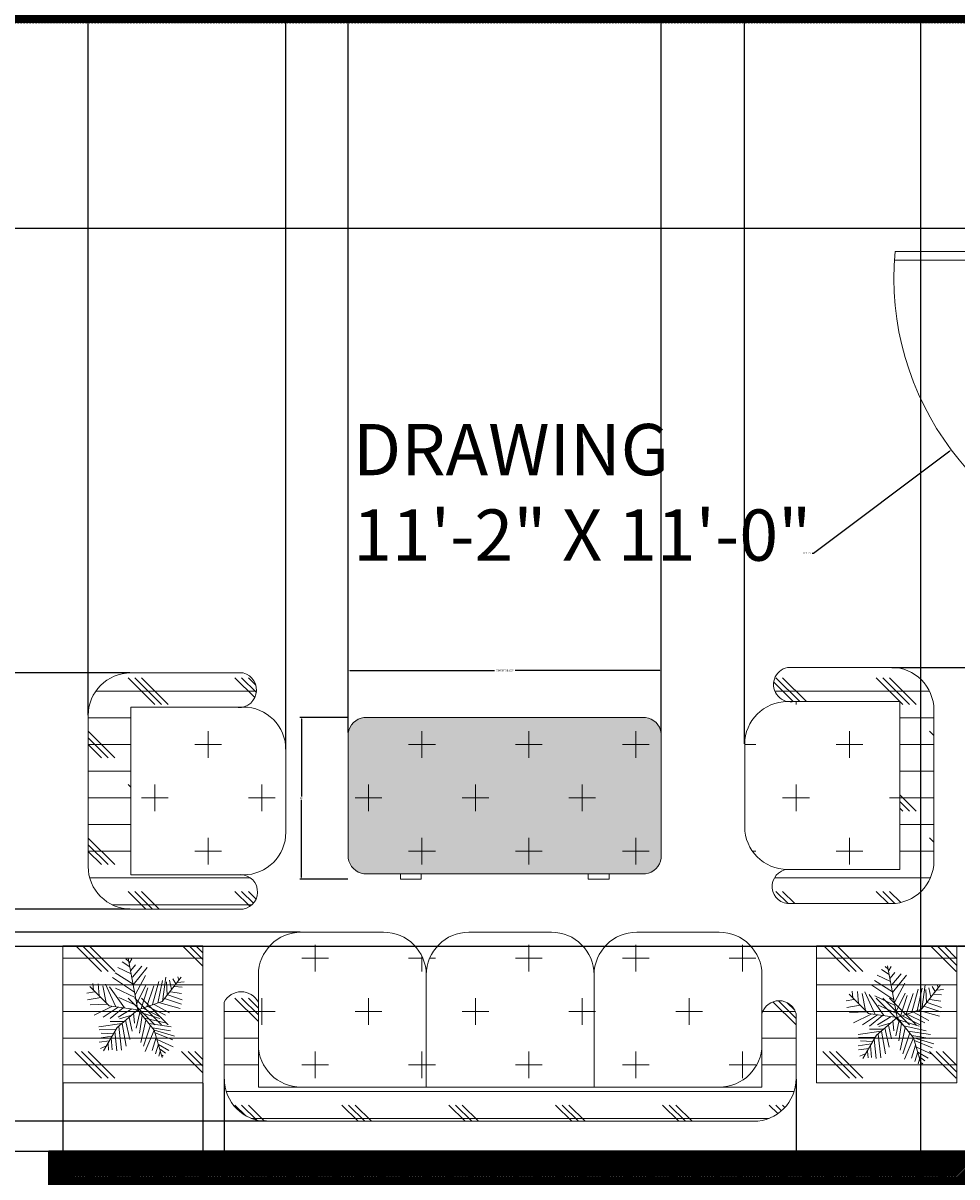
# Model space of a CAD drawing. Units: inches. Extents: x 557 to 1007, y 390 to 953.
# Tile 6 of 10: x 842 to 952, y 612 to 747. Entities that reach past the tile are written whole.
import ezdxf

# ---------------------------------------------------------------- set-up
doc = ezdxf.new("R2010")
doc.units = ezdxf.units.IN
doc.header["$LTSCALE"] = 5
doc.header["$MEASUREMENT"] = 0
for name, color, linetype, lineweight in [('A-ANNO-DIMS', 2, 'Continuous', 18), ('A-AREA-IDEN', 7, 'Continuous', 18), ('A-DOOR', 3, 'Continuous', 18), ('A-FURN', 8, 'Continuous', 18), ('A-FURN-PATT', 9, 'Continuous', 9), ('A-WALL', 7, 'Continuous', 35)]:
    doc.layers.add(name, color=color, linetype=linetype, lineweight=lineweight)
doc.layers.add('A-GLAZ-PATT', color=141, linetype='Continuous', lineweight=9, true_color=0xadddf7)
doc.layers.add('A-WALL-PATT', color=251, linetype='Continuous', lineweight=9, true_color=0x636466)
doc.styles.get("Standard").update_dxf_attribs({"font": 'arial.ttf'})
doc.dimstyles.get("Standard").update_dxf_attribs({"dimtxt": 0.18, "dimasz": 0.18, "dimexe": 0.18, "dimexo": 0.0625, "dimgap": 0.09, "dimtad": 0, "dimtih": 1, "dimtoh": 1, "dimdec": 4, "dimzin": 0, "dimdsep": 46, "dimtxsty": 'Standard', "dimcen": 0.09, "dimadec": 0, "dimazin": 0, "dimtfac": 1, "dimtdec": 4, "dimtofl": 0, "dimtmove": 0, "dimatfit": 3, "dimfxl": 1, "dimtolj": 1, "dimtzin": 0, "dimarcsym": 0})

# ---------------------------------------------------------------- blocks, each defined once
blk = doc.blocks.new('*U13')
for p, q in [((-8.737, 47.138), (-17.069, 52.711)), ((-10.186, 53.64), (-13.084, 55.962)), ((0, 0), (-10.5, 57)), ((-9.099, 51.782), (-6.563, 55.962)), ((-5.114, 28.097), (-24.676, 40.636)), ((-7.288, 39.707), (-21.778, 46.673)), ((-7.65, 43.423), (-2.578, 49.46)), ((-5.839, 35.992), (4.667, 48.067)), ((-5.114, 27.632), (10.463, 46.673)), ((-31.5, 4.5), (-52.5, 25.5)), ((-48.585, 21.131), (-49.309, 29.026)), ((-43.513, 28.561), (-42.427, 15.558)), ((-38.442, 26.239), (-34.819, 7.663)), ((-35.544, 28.097), (-24.314, 3.947)), ((-3.665, 19.273), (-27.574, 35.527)), ((-2.941, 16.486), (8.652, 37.85)), ((-1.129, 6.734), (9.014, 26.704)), ((10.101, 3.483), (17.708, 26.239)), ((16.259, 5.805), (23.142, 31.348)), ((22.055, 7.198), (27.489, 32.277)), ((27, 9), (48, 36)), ((27.127, 9.056), (31.112, 35.992)), ((31.836, 30.883), (32.561, 16.486)), ((35.096, 32.741), (37.27, 22.524)), ((38.719, 34.134), (41.979, 28.561)), ((40.53, 25.775), (48.862, 24.846)), ((43.791, 29.954), (51.036, 30.883)), ((44.153, 36.456), (45.239, 32.741)), ((-47.498, 19.737), (-55.83, 18.344)), ((-40.615, 13.7), (-55.105, 10.913)), ((-14.533, 2.09), (-30.834, 25.31)), ((-24.314, 23.917), (-2.941, 13.7)), ((-20.691, 13.7), (-1.129, 4.876)), ((3.942, 1.625), (11.187, 24.381)), ((33.285, 16.486), (48.862, 10.913)), ((36.183, 19.737), (48.137, 17.88)), ((-33.37, 6.269), (-52.207, 5.34)), ((-28.299, 3.483), (-47.86, -5.805)), ((-21.416, 3.018), (-38.079, -8.128)), ((0, 0), (-31.5, 4.5)), ((-15.982, 2.09), (-30.11, -9.521)), ((0, 0), (-22.5, -19.5)), ((-6.563, 1.161), (-21.416, -8.128)), ((0, 0), (27, 9)), ((0, 0), (18, -22.5)), ((6.478, 1.625), (26.04, -8.592)), ((11.187, 3.483), (30.749, -5.805)), ((18.07, 5.805), (35.096, -3.483)), ((24.229, 7.663), (46.688, 1.625)), ((29.662, 12.307), (48.137, 6.269)), ((-6.563, -5.805), (-19.967, -9.985)), ((-13.446, -11.378), (-8.737, -32.741)), ((-9.461, -8.592), (-6.201, -23.453)), ((-4.752, -3.483), (-3.665, -14.629)), ((2.493, -3.019), (-1.491, -20.202)), ((1.769, -2.555), (24.229, -9.521)), ((5.029, -6.27), (2.131, -25.775)), ((9.014, -11.378), (3.58, -35.992)), ((7.565, -9.056), (32.198, -14.629)), ((-17.431, -15.094), (-42.789, -18.809)), ((-24.314, -21.596), (-42.427, -22.06)), ((-22.5, -19.5), (-37.5, -45)), ((-15.257, -12.772), (-30.11, -12.772)), ((-25.038, -23.918), (-22.865, -45.281)), ((-20.691, -18.345), (-17.793, -44.352)), ((-17.069, -15.094), (-12.721, -40.172)), ((14.085, -16.951), (6.478, -40.172)), ((18.07, -22.524), (8.289, -45.745)), ((12.274, -15.094), (36.907, -18.809)), ((16.259, -19.738), (36.183, -22.989)), ((18, -22.5), (27, -52.5)), ((18.433, -22.524), (40.53, -29.026)), ((19.157, -25.311), (38.719, -33.206)), ((-28.299, -29.026), (-42.789, -31.348)), ((-30.834, -34.135), (-42.427, -35.528)), ((-26.849, -26.24), (-40.253, -25.775)), ((-32.646, -36.921), (-31.921, -44.352)), ((-29.023, -30.884), (-27.936, -43.887)), ((20.244, -30.419), (15.897, -44.816)), ((22.78, -37.85), (19.519, -48.532)), ((21.331, -32.741), (39.081, -40.636)), ((-34.457, -39.708), (-40.978, -42.494)), ((22.78, -38.314), (34.372, -44.816)), ((24.591, -45.745), (23.142, -50.854)), ((24.591, -43.423), (30.749, -47.603)), ((26.764, -49.925), (28.213, -50.854))]:
    blk.add_line(p, q)
blk = doc.blocks.new('Desk - 30 x 60 in.')
for p, q in [((-26.999995, 0), (26.999995, 0)), ((-29.999995, -27), (-29.999995, -3)), ((29.999995, -3), (29.999995, -27)), ((26.999995, -30), (-26.999995, -30)), ((-20.000005, -30), (-20.000005, -31)), ((-16.000005, -31), (-16.000005, -30)), ((15.999995, -31), (15.999995, -30)), ((19.999995, -30), (19.999995, -31)), ((-20.000005, -31), (-16.000005, -31)), ((19.999995, -31), (15.999995, -31))]:
    blk.add_line(p, q)
for centre, start, end in [((-26.499995, -3.5), 98.1301, 171.8699), ((26.499995, -3.5), 8.130102, 81.8699), ((-26.499995, -26.5), 188.1301, 261.8699), ((26.499995, -26.5), 278.1301, 351.8699)]:
    blk.add_arc(centre, 3.535534, start, end)
blk = doc.blocks.new('*D43')
at = {"layer": 'A-ANNO-DIMS', "color": 0, "lineweight": -2, "ltscale": 5, "transparency": 16777216}
for p, q in [((880.45, 665.73), (880.45, 671.34)), ((880.63, 671.16), (897.55, 671.16)), ((916.87, 671.16), (899.95, 671.16)), ((917.05, 665.73), (917.05, 671.34))]:
    blk.add_line(p, q, dxfattribs=at)
at = {"layer": 'A-ANNO-DIMS', "color": 0, "ltscale": 5, "transparency": 16777216}
for points in [[(880.63, 671.19), (880.63, 671.13), (880.45, 671.16)], [(916.87, 671.19), (916.87, 671.13), (917.05, 671.16)]]:
    blk.add_solid(points, dxfattribs=at)
at = {"layer": 'Defpoints', "color": 0, "ltscale": 5, "transparency": 16777216}
for p in [(917.05, 671.16), (880.45, 665.67), (917.05, 665.67)]:
    blk.add_point(p, dxfattribs=at)
at = {"layer": 'A-ANNO-DIMS', "color": 0, "ltscale": 5, "transparency": 16777216, "insert": (898.75, 671.16), "char_height": 0.18, "attachment_point": 5}
blk.add_mtext('\\A1;CENTER TABLE 37', dxfattribs=at)
blk = doc.blocks.new('*D44')
at = {"layer": 'A-ANNO-DIMS', "color": 0, "lineweight": -2, "ltscale": 5, "transparency": 16777216}
for p, q in [((880.39, 665.67), (874.78, 665.67)), ((874.96, 665.49), (874.96, 656.4)), ((874.96, 646.94), (874.96, 656.03)), ((880.39, 646.76), (874.78, 646.76))]:
    blk.add_line(p, q, dxfattribs=at)
at = {"layer": 'A-ANNO-DIMS', "color": 0, "ltscale": 5, "transparency": 16777216}
for points in [[(874.93, 665.49), (874.99, 665.49), (874.96, 665.67)], [(874.93, 646.94), (874.99, 646.94), (874.96, 646.76)]]:
    blk.add_solid(points, dxfattribs=at)
at = {"layer": 'Defpoints', "color": 0, "ltscale": 5, "transparency": 16777216}
for p in [(874.96, 665.67), (880.45, 665.67), (880.45, 646.76)]:
    blk.add_point(p, dxfattribs=at)
at = {"layer": 'A-ANNO-DIMS', "color": 0, "ltscale": 5, "transparency": 16777216, "insert": (874.96, 656.22), "char_height": 0.18, "attachment_point": 5}
blk.add_mtext('\\A1;19', dxfattribs=at)
blk = doc.blocks.new('*D60')
at = {"layer": 'A-ANNO-DIMS', "color": 0, "lineweight": -2, "ltscale": 5, "transparency": 16777216}
for p, q in [((683.47, 722.9), (1006.54, 722.9)), ((1006.36, 722.72), (1006.36, 681.09)), ((1006.36, 639.08), (1006.36, 680.72)), ((683.47, 638.9), (1006.54, 638.9))]:
    blk.add_line(p, q, dxfattribs=at)
at = {"layer": 'A-ANNO-DIMS', "color": 0, "ltscale": 5, "transparency": 16777216}
for points in [[(1006.33, 722.72), (1006.39, 722.72), (1006.36, 722.9)], [(1006.33, 639.08), (1006.39, 639.08), (1006.36, 638.9)]]:
    blk.add_solid(points, dxfattribs=at)
at = {"layer": 'Defpoints', "color": 0, "ltscale": 5, "transparency": 16777216}
for p in [(683.41, 722.9), (683.41, 638.9), (1006.36, 638.9)]:
    blk.add_point(p, dxfattribs=at)
at = {"layer": 'A-ANNO-DIMS', "color": 0, "ltscale": 5, "transparency": 16777216, "insert": (1006.36, 680.9), "char_height": 0.18, "attachment_point": 5}
blk.add_mtext('\\A1;84', dxfattribs=at)
blk = doc.blocks.new('*D61')
at = {"layer": 'A-ANNO-DIMS', "color": 0, "lineweight": -2, "ltscale": 5, "transparency": 16777216}
for p, q in [((683.47, 638.9), (1006.54, 638.9)), ((1006.36, 638.72), (1006.36, 627.08)), ((1006.36, 615.08), (1006.36, 626.72)), ((683.47, 614.9), (1006.54, 614.9))]:
    blk.add_line(p, q, dxfattribs=at)
at = {"layer": 'A-ANNO-DIMS', "color": 0, "ltscale": 5, "transparency": 16777216}
for points in [[(1006.33, 638.72), (1006.39, 638.72), (1006.36, 638.9)], [(1006.33, 615.08), (1006.39, 615.08), (1006.36, 614.9)]]:
    blk.add_solid(points, dxfattribs=at)
at = {"layer": 'Defpoints', "color": 0, "ltscale": 5, "transparency": 16777216}
for p in [(683.41, 638.9), (683.41, 614.9), (1006.36, 614.9)]:
    blk.add_point(p, dxfattribs=at)
at = {"layer": 'A-ANNO-DIMS', "color": 0, "ltscale": 5, "transparency": 16777216, "insert": (1006.36, 626.9), "char_height": 0.18, "attachment_point": 5}
blk.add_mtext('\\A1;24', dxfattribs=at)
blk = doc.blocks.new('*D80')
at = {"layer": 'A-ANNO-DIMS', "color": 0, "lineweight": -2, "ltscale": 5, "transparency": 16777216}
for p, q in [((865.93, 623.35), (865.93, 597.28)), ((932.83, 623.35), (932.83, 597.28)), ((866.11, 597.46), (899.06, 597.46)), ((932.65, 597.46), (899.71, 597.46))]:
    blk.add_line(p, q, dxfattribs=at)
at = {"layer": 'A-ANNO-DIMS', "color": 0, "ltscale": 5, "transparency": 16777216}
for points in [[(866.11, 597.49), (866.11, 597.43), (865.93, 597.46)], [(932.65, 597.49), (932.65, 597.43), (932.83, 597.46)]]:
    blk.add_solid(points, dxfattribs=at)
at = {"layer": 'Defpoints', "color": 0, "ltscale": 5, "transparency": 16777216}
for p in [(865.93, 623.41), (932.83, 623.41), (865.93, 597.46)]:
    blk.add_point(p, dxfattribs=at)
at = {"layer": 'A-ANNO-DIMS', "color": 0, "ltscale": 5, "transparency": 16777216, "insert": (899.38, 597.46), "char_height": 0.18, "attachment_point": 5}
blk.add_mtext('\\A1;66.9', dxfattribs=at)
blk = doc.blocks.new('*D81')
at = {"layer": 'A-ANNO-DIMS', "color": 0, "lineweight": -2, "ltscale": 5, "transparency": 16777216}
for p, q in [((874.87, 640.54), (556.69, 640.54)), ((556.87, 640.36), (556.87, 629.66)), ((556.87, 618.59), (556.87, 629.29)), ((870.87, 618.41), (556.69, 618.41))]:
    blk.add_line(p, q, dxfattribs=at)
at = {"layer": 'A-ANNO-DIMS', "color": 0, "ltscale": 5, "transparency": 16777216}
for points in [[(556.84, 640.36), (556.9, 640.36), (556.87, 640.54)], [(556.84, 618.59), (556.9, 618.59), (556.87, 618.41)]]:
    blk.add_solid(points, dxfattribs=at)
at = {"layer": 'Defpoints', "color": 0, "ltscale": 5, "transparency": 16777216}
for p in [(874.93, 640.54), (556.87, 618.41), (870.93, 618.41)]:
    blk.add_point(p, dxfattribs=at)
at = {"layer": 'A-ANNO-DIMS', "color": 0, "ltscale": 5, "transparency": 16777216, "insert": (556.87, 629.48), "char_height": 0.18, "attachment_point": 5}
blk.add_mtext('\\A1;22.13', dxfattribs=at)
blk = doc.blocks.new('*D82')
at = {"layer": 'A-ANNO-DIMS', "color": 0, "lineweight": -2, "ltscale": 5, "transparency": 16777216}
for p, q in [((850.01, 665.94), (850.01, 953.03)), ((850.19, 952.85), (861.18, 952.85)), ((872.97, 952.85), (861.98, 952.85)), ((873.15, 661.94), (873.15, 953.03))]:
    blk.add_line(p, q, dxfattribs=at)
at = {"layer": 'A-ANNO-DIMS', "color": 0, "ltscale": 5, "transparency": 16777216}
for points in [[(850.19, 952.88), (850.19, 952.82), (850.01, 952.85)], [(872.97, 952.88), (872.97, 952.82), (873.15, 952.85)]]:
    blk.add_solid(points, dxfattribs=at)
at = {"layer": 'Defpoints', "color": 0, "ltscale": 5, "transparency": 16777216}
for p in [(873.15, 952.85), (850.01, 665.88), (873.15, 661.88)]:
    blk.add_point(p, dxfattribs=at)
at = {"layer": 'A-ANNO-DIMS', "color": 0, "ltscale": 5, "transparency": 16777216, "insert": (861.58, 952.85), "char_height": 0.18, "attachment_point": 5}
blk.add_mtext('\\A1;23.13', dxfattribs=at)
blk = doc.blocks.new('*D83')
at = {"layer": 'A-ANNO-DIMS', "color": 0, "lineweight": -2, "ltscale": 5, "transparency": 16777216}
for p, q in [((854.95, 670.88), (828.88, 670.88)), ((829.06, 670.7), (829.06, 657.24)), ((829.06, 643.42), (829.06, 656.88)), ((854.95, 643.24), (828.88, 643.24))]:
    blk.add_line(p, q, dxfattribs=at)
at = {"layer": 'A-ANNO-DIMS', "color": 0, "ltscale": 5, "transparency": 16777216}
for points in [[(829.03, 670.7), (829.09, 670.7), (829.06, 670.88)], [(829.03, 643.42), (829.09, 643.42), (829.06, 643.24)]]:
    blk.add_solid(points, dxfattribs=at)
at = {"layer": 'Defpoints', "color": 0, "ltscale": 5, "transparency": 16777216}
for p in [(829.06, 670.88), (855.01, 670.88), (855.01, 643.24)]:
    blk.add_point(p, dxfattribs=at)
at = {"layer": 'A-ANNO-DIMS', "color": 0, "ltscale": 5, "transparency": 16777216, "insert": (829.06, 657.06), "char_height": 0.18, "attachment_point": 5}
blk.add_mtext('\\A1;27.634', dxfattribs=at)
blk = doc.blocks.new('*D84')
at = {"layer": 'A-ANNO-DIMS', "color": 0, "lineweight": -2, "ltscale": 5, "transparency": 16777216}
for p, q in [((847.04, 622.86), (847.04, 389.77)), ((863.45, 622.86), (863.45, 389.77)), ((847.22, 389.95), (854.79, 389.95)), ((863.27, 389.95), (855.7, 389.95))]:
    blk.add_line(p, q, dxfattribs=at)
at = {"layer": 'A-ANNO-DIMS', "color": 0, "ltscale": 5, "transparency": 16777216}
for points in [[(847.22, 389.98), (847.22, 389.92), (847.04, 389.95)], [(863.27, 389.98), (863.27, 389.92), (863.45, 389.95)]]:
    blk.add_solid(points, dxfattribs=at)
at = {"layer": 'Defpoints', "color": 0, "ltscale": 5, "transparency": 16777216}
for p in [(847.04, 622.92), (863.45, 622.92), (863.45, 389.95)]:
    blk.add_point(p, dxfattribs=at)
at = {"layer": 'A-ANNO-DIMS', "color": 0, "ltscale": 5, "transparency": 16777216, "insert": (855.24, 389.95), "char_height": 0.18, "attachment_point": 5}
blk.add_mtext('\\A1;16.408', dxfattribs=at)
blk = doc.blocks.new('*D86')
at = {"layer": 'A-ANNO-DIMS', "color": 0, "lineweight": -2, "ltscale": 5, "transparency": 16777216}
for p, q in [((873.15, 661.94), (873.15, 953.03)), ((873.33, 952.85), (876.4, 952.85)), ((880.27, 952.85), (877.19, 952.85)), ((880.45, 663.9), (880.45, 953.03))]:
    blk.add_line(p, q, dxfattribs=at)
at = {"layer": 'A-ANNO-DIMS', "color": 0, "ltscale": 5, "transparency": 16777216}
for points in [[(873.33, 952.88), (873.33, 952.82), (873.15, 952.85)], [(880.27, 952.88), (880.27, 952.82), (880.45, 952.85)]]:
    blk.add_solid(points, dxfattribs=at)
at = {"layer": 'Defpoints', "color": 0, "ltscale": 5, "transparency": 16777216}
for p in [(880.45, 952.85), (880.45, 663.84), (873.15, 661.88)]:
    blk.add_point(p, dxfattribs=at)
at = {"layer": 'A-ANNO-DIMS', "color": 0, "ltscale": 5, "transparency": 16777216, "insert": (876.8, 952.85), "char_height": 0.18, "attachment_point": 5}
blk.add_mtext('\\A1;7.303', dxfattribs=at)
blk = doc.blocks.new('*D87')
at = {"layer": 'A-ANNO-DIMS', "color": 0, "lineweight": -2, "ltscale": 5, "transparency": 16777216}
for p, q in [((917.05, 663.9), (917.05, 953.03)), ((917.23, 952.85), (921.61, 952.85)), ((926.63, 952.85), (922.26, 952.85)), ((926.81, 662.58), (926.81, 953.03))]:
    blk.add_line(p, q, dxfattribs=at)
at = {"layer": 'A-ANNO-DIMS', "color": 0, "ltscale": 5, "transparency": 16777216}
for points in [[(917.23, 952.88), (917.23, 952.82), (917.05, 952.85)], [(926.63, 952.88), (926.63, 952.82), (926.81, 952.85)]]:
    blk.add_solid(points, dxfattribs=at)
at = {"layer": 'Defpoints', "color": 0, "ltscale": 5, "transparency": 16777216}
for p in [(926.81, 952.85), (917.05, 663.84), (926.81, 662.52)]:
    blk.add_point(p, dxfattribs=at)
at = {"layer": 'A-ANNO-DIMS', "color": 0, "ltscale": 5, "transparency": 16777216, "insert": (921.93, 952.85), "char_height": 0.18, "attachment_point": 5}
blk.add_mtext('\\A1;9.76', dxfattribs=at)
blk = doc.blocks.new('*D88')
at = {"layer": 'A-ANNO-DIMS', "color": 0, "lineweight": -2, "ltscale": 5, "transparency": 16777216}
for p, q in [((944.01, 671.52), (1006.54, 671.52)), ((1006.36, 671.34), (1006.36, 655.41)), ((1006.36, 639.12), (1006.36, 655.05)), ((951.7, 638.94), (1006.54, 638.94))]:
    blk.add_line(p, q, dxfattribs=at)
at = {"layer": 'A-ANNO-DIMS', "color": 0, "ltscale": 5, "transparency": 16777216}
for points in [[(1006.33, 671.34), (1006.39, 671.34), (1006.36, 671.52)], [(1006.33, 639.12), (1006.39, 639.12), (1006.36, 638.94)]]:
    blk.add_solid(points, dxfattribs=at)
at = {"layer": 'Defpoints', "color": 0, "ltscale": 5, "transparency": 16777216}
for p in [(943.95, 671.52), (951.64, 638.94), (1006.36, 638.94)]:
    blk.add_point(p, dxfattribs=at)
at = {"layer": 'A-ANNO-DIMS', "color": 0, "ltscale": 5, "transparency": 16777216, "insert": (1006.36, 655.23), "char_height": 0.18, "attachment_point": 5}
blk.add_mtext('\\A1;32.58', dxfattribs=at)
blk = doc.blocks.new('*D96')
at = {"layer": 'A-ANNO-DIMS', "color": 0, "lineweight": -2, "ltscale": 5, "transparency": 16777216}
for p, q in [((947.41, 536.97), (947.41, 953.03)), ((947.59, 952.85), (959.19, 952.85)), ((971.23, 952.85), (959.63, 952.85)), ((971.41, 512.97), (971.41, 953.03))]:
    blk.add_line(p, q, dxfattribs=at)
at = {"layer": 'A-ANNO-DIMS', "color": 0, "ltscale": 5, "transparency": 16777216}
for points in [[(947.59, 952.88), (947.59, 952.82), (947.41, 952.85)], [(971.23, 952.88), (971.23, 952.82), (971.41, 952.85)]]:
    blk.add_solid(points, dxfattribs=at)
at = {"layer": 'Defpoints', "color": 0, "ltscale": 5, "transparency": 16777216}
for p in [(971.41, 952.85), (947.41, 536.9), (971.41, 512.9)]:
    blk.add_point(p, dxfattribs=at)
at = {"layer": 'A-ANNO-DIMS', "color": 0, "ltscale": 5, "transparency": 16777216, "insert": (959.41, 952.85), "char_height": 0.18, "attachment_point": 5}
blk.add_mtext('\\A1;24', dxfattribs=at)
blk = doc.blocks.new('*D105')
at = {"layer": 'A-ANNO-DIMS', "color": 0, "lineweight": -2, "ltscale": 5, "transparency": 16777216}
for p, q in [((977.72, 717.11), (977.9, 717.11)), ((977.81, 717.02), (977.81, 717.2)), ((934.87, 684.9), (950.83, 696.87)), ((934.69, 684.9), (934.87, 684.9))]:
    blk.add_line(p, q, dxfattribs=at)
at = {"layer": 'A-ANNO-DIMS', "color": 0, "ltscale": 5, "transparency": 16777216}
blk.add_solid([(950.81, 696.9), (950.85, 696.85), (950.97, 696.98)], dxfattribs=at)
at = {"layer": 'Defpoints', "color": 0, "ltscale": 5, "transparency": 16777216}
for p in [(977.81, 717.11), (950.97, 696.98)]:
    blk.add_point(p, dxfattribs=at)
at = {"layer": 'A-ANNO-DIMS', "color": 0, "ltscale": 5, "transparency": 16777216, "insert": (934.14, 684.9), "char_height": 0.18, "attachment_point": 5}
blk.add_mtext('\\A1;R33.545', dxfattribs=at)

msp = doc.modelspace()

# ---------------------------------------------------------------- hatches: boundary and pattern name
at = {"layer": 'A-FURN-PATT', "ltscale": 5}
h = msp.add_hatch(dxfattribs=at)
h.set_pattern_fill('GRAVEL', color=256, scale=25)
h.set_pattern_definition([(228.01279, (18, 25), (-200, -225), [3.3634, -332.9772]), (184.96974, (15.75, 22.5), (300, 25), [5.7717, -571.39812]), (132.51045, (10, 22), (250, -275), [4.0697, -402.9008]), (267.27369, (0.25, 15.75), (25, 500), [5.25595, -520.33895]), (292.83365, (0, 10.5), (-125, 300), [5.15387, -510.23433]), (357.27369, (2, 5.75), (-500, 25), [5.25595, -520.33895]), (37.69424, (7.25, 5.5), (-325, -250), [6.95072, -688.1212]), (72.25533, (12.75, 9.75), (175, 550), [6.5622, -649.65804]), (121.42957, (14.75, 16), (-200, 325), [5.27375, -522.10183]), (175.23636, (12, 20.5), (275, -25), [6.0208, -295.01906]), (222.39744, (6, 21), (-300, -275), [7.7862, -770.83438]), (138.81407, (25, 15.5), (-175, 150), [2.65752, -263.0961]), (171.46923, (23, 17.25), (325, -50), [5.05593, -500.5378]), (225, (18, 18), (-3e-15, -25), [3.53552, -31.8198]), (203.1986, (16.25, 21), (125, 50), [1.90395, -188.49038]), (291.8014, (14.5, 20.25), (-25, 75), [2.69257, -131.93655]), (30.96376, (15.5, 17.75), (75, 50), [4.37322, -141.40057]), (161.56505, (19.25, 20), (50, -25), [3.16228, -75.89467]), (16.38954, (0, 20.25), (250, 75), [4.43, -438.57113]), (70.34618, (4.25, 21.5), (-100, -275), [3.71652, -367.9352]), (293.1986, (19.25, 25), (-50, 125), [3.80788, -186.58645]), (343.61046, (20.75, 21.5), (-250, 75), [4.43, -438.57113]), (339.44395, (0, 4.75), (-125, 50), [4.272, -209.3281]), (294.77514, (4, 3.25), (-125, 275), [3.57945, -354.36608]), (66.8014, (19.5, 0), (50, 125), [3.80788, -186.58645]), (17.35402, (21, 3.5), (-325, -100), [4.19078, -414.8856]), (69.44395, (7.25, 0), (-50, -125), [2.136, -211.4641]), (101.30993, (18, 0), (-25, 100), [1.27475, -126.20074]), (165.96376, (17.75, 1.25), (75, -25), [5.15388, -97.92377]), (186.00901, (12.75, 2.5), (250, 25), [4.77625, -472.84808]), (303.69007, (15.5, 15.5), (-25, 50), [3.60555, -86.53323]), (353.15723, (17.5, 12.5), (425, -50), [6.29485, -623.18907]), (60.9454, (23.75, 11.75), (-100, -175), [2.5739, -254.81685]), (90, (25, 14), (-25, 25), [1.5, -23.5]), (120.25644, (12.25, 3.25), (100, -175), [3.4731, -343.838]), (48.01279, (10.5, 6.25), (200, 225), [6.7268, -329.6138]), (0, (15, 11.25), (25, 25), [6.5, -18.5]), (325.30485, (21.5, 11.25), (250, -175), [3.95285, -391.33186]), (254.0546, (24.75, 9), (-25, -100), [3.64005, -178.3627]), (207.64598, (23.75, 5.5), (-475, -250), [5.92662, -586.73685]), (175.42608, (18.5, 2.75), (-325, 25), [6.26997, -620.72684])])
h.paths.add_polyline_path([(615.2525, 688.5, 1), (640.7475, 688.5, 1)])
h.paths.add_polyline_path([(917.0544, 663.8414, 0.33333323), (915.2241, 665.6717), (882.2793, 665.6717, 0.33333323), (880.449, 663.8414), (880.449, 649.1992, 0.33333323), (882.2793, 647.369), (915.2241, 647.369, 0.33333323), (917.0544, 649.1992)])
h.paths.add_polyline_path([(828.0807, 699.7098), (756.0807, 699.7098), (756.0807, 663.7098), (828.0807, 663.7098)])
h.paths.add_polyline_path([(787.5651, 663.7098), (768.5964, 663.7098), (769.8463, 655.7098), (786.3151, 655.7098)])
h.paths.add_polyline_path([(815.5651, 663.7098), (796.5964, 663.7098), (797.8463, 655.7098), (814.3151, 655.7098)])
h.paths.add_polyline_path([(836.0807, 689.9442), (828.0807, 691.1942), (828.0807, 672.2255), (836.0807, 673.4755)])
h.paths.add_polyline_path([(756.0807, 691.1942), (748.0807, 689.9442), (748.0807, 673.4755), (756.0807, 672.2255)])
h.paths.add_polyline_path([(786.3151, 707.7098), (769.8463, 707.7098), (768.5964, 699.7098), (787.5651, 699.7098)])
h.paths.add_polyline_path([(814.3151, 707.7098), (797.8463, 707.7098), (796.5964, 699.7098), (815.5651, 699.7098)])
h.paths.add_polyline_path([(917.4362, 607.3575), (889.5896, 607.3575), (889.5896, 586.4726), (917.4362, 586.4726)])
h.paths.add_polyline_path([(721.4053, 881.8539), (671.0053, 881.8539), (671.0053, 866.6539), (658.2053, 866.6539), (658.2053, 821.8539), (721.4053, 821.8539)])
h.paths.add_polyline_path([(925.4053, 875.1046), (875.0053, 875.1046), (875.0053, 859.9046), (862.2053, 859.9046), (862.2053, 815.1046), (925.4053, 815.1046)])
h.paths.add_polyline_path([(721.4053, 558.9046), (671.0053, 558.9046), (671.0053, 543.7046), (658.2053, 543.7046), (658.2053, 498.9046), (721.4053, 498.9046)])
at = {"layer": 'A-FURN-PATT'}
h = msp.add_hatch(dxfattribs=at)
h.set_pattern_fill('CROSS', color=256, scale=25)
h.paths.add_polyline_path([(925.4053, 875.1046), (875.0053, 875.1046), (875.0053, 859.9046), (862.2053, 859.9046), (862.2053, 815.1046), (925.4053, 815.1046)])
h.paths.add_polyline_path([(721.4053, 881.8539), (671.0053, 881.8539), (671.0053, 866.6539), (658.2053, 866.6539), (658.2053, 821.8539), (721.4053, 821.8539)])
h.paths.add_polyline_path([(671.0053, 881.8539), (655.8053, 866.6539), (671.0053, 866.6539)], flags=17)
h.paths.add_polyline_path([(671.0053, 881.8539), (641.4053, 881.8539), (641.4053, 821.8539), (655.8053, 821.8539), (655.8053, 829.8539), (642.6053, 829.8539), (642.6053, 850.6539), (655.8053, 850.6539), (655.8053, 853.0539), (642.6053, 853.0539), (642.6053, 873.8539), (657.8053, 873.8539), (657.8053, 868.6539)])
h.paths.add_polyline_path([(875.0053, 875.1046), (859.8053, 859.9046), (875.0053, 859.9046)], flags=17)
h.paths.add_polyline_path([(875.0053, 875.1046), (845.4053, 875.1046), (845.4053, 815.1046), (859.8053, 815.1046), (859.8053, 823.1046), (846.6053, 823.1046), (846.6053, 843.9046), (859.8053, 843.9046), (859.8053, 846.3046), (846.6053, 846.3046), (846.6053, 867.1046), (861.8053, 867.1046), (861.8053, 861.9046)])
h.paths.add_polyline_path([(721.4053, 558.9046), (671.0053, 558.9046), (671.0053, 543.7046), (658.2053, 543.7046), (658.2053, 498.9046), (721.4053, 498.9046)])
h.paths.add_polyline_path([(671.0053, 558.9046), (641.4053, 558.9046), (641.4053, 498.9046), (655.8053, 498.9046), (655.8053, 506.9046), (642.6053, 506.9046), (642.6053, 527.7046), (655.8053, 527.7046), (655.8053, 530.1046), (642.6053, 530.1046), (642.6053, 550.9046), (657.8053, 550.9046), (657.8053, 545.7046)])
h.paths.add_polyline_path([(671.0053, 558.9046), (657.8053, 545.7046), (655.8053, 543.7046), (671.0053, 543.7046)], flags=17)
h.paths.add_polyline_path([(873.1461, 661.8773, 0.41421356), (868.1461, 666.8773, -0.12244426), (867.1516, 666.8773), (855.014, 666.8773), (855.014, 647.2429), (867.4581, 647.2429, -0.08537395), (868.1461, 647.2429, 0.41421356), (873.1461, 652.2429)])
h.paths.add_polyline_path([(917.0544, 663.8414, 0.33333323), (915.2241, 665.6717), (882.2793, 665.6717, 0.33333323), (880.449, 663.8414), (880.449, 649.1992, 0.33333323), (882.2793, 647.369), (915.2241, 647.369, 0.33333323), (917.0544, 649.1992)])
h.paths.add_polyline_path([(944.9465, 667.5202), (932.6561, 667.5202, -0.10407786), (931.8144, 667.5202, 0.41421356), (926.8144, 662.5202), (926.8144, 652.8858, 0.41421356), (931.8144, 647.8858, -0.05611627), (932.2647, 647.8858), (944.9465, 647.8858)])
h.paths.add_polyline_path([(928.8341, 635.542, 0.41421356), (923.8341, 640.542), (914.1997, 640.542, 0.41421356), (909.1997, 635.542), (909.1997, 622.4099), (923.8341, 622.4099, 0.41421356), (928.8341, 627.4099)])
h.paths.add_polyline_path([(909.1997, 635.542, 0.41421356), (904.1997, 640.542), (894.5653, 640.542, 0.41421356), (889.5653, 635.542), (889.5653, 622.4099), (909.1997, 622.4099)])
h.paths.add_polyline_path([(889.5653, 635.542, 0.41421356), (884.5653, 640.542), (874.9308, 640.542, 0.41421356), (869.9308, 635.542), (869.9308, 627.4099, 0.41421356), (874.9308, 622.4099), (889.5653, 622.4099)])
h = msp.add_hatch(dxfattribs=at)
h.set_pattern_fill('CORK', color=256, scale=25)
h.set_pattern_definition([(0, (0, 0), (0, 3.125), []), (135, (1.5625, -1.5625), (-6.25, -6.25), [4.41942, -4.41942]), (135, (2.344, -1.5625), (-6.25, -6.25), [4.41942, -4.41942]), (135, (3.125, -1.5625), (-6.25, -6.25), [4.41942, -4.41942])])
h.paths.add_polyline_path([(932.8341, 623.4099), (932.8341, 630.9869, 0.76666915), (928.8341, 630.9869), (928.8341, 627.4099), (928.8341, 622.4099), (909.1997, 622.4099), (874.9308, 622.4099), (869.9308, 622.4099), (869.9308, 632.3614, 0.60407544), (865.9308, 632.3614), (865.9308, 623.4099, 0.41421356), (870.9308, 618.4099), (927.8341, 618.4099, 0.41421356)])
h.paths.add_polyline_path([(855.014, 666.8773), (868.1461, 666.8773, 0.78182568), (868.1461, 670.8773), (855.014, 670.8773, 0.41421356), (850.014, 665.8773), (850.014, 648.2429, 0.41421356), (855.014, 643.2429), (868.1461, 643.2429, 0.84268288), (868.1461, 647.2429), (855.014, 647.2429)])
h.paths.add_polyline_path([(948.9465, 666.5202, 0.41421356), (943.9465, 671.5202), (931.8144, 671.5202, 0.81146646), (931.8144, 667.5202), (944.9465, 667.5202), (944.9465, 647.8858), (931.8144, 647.8858, 0.89373088), (931.8144, 643.8858), (943.9465, 643.8858, 0.41421356), (948.9465, 648.8858)])
h.paths.add_polyline_path([(951.6399, 638.9424), (935.2317, 638.9424), (935.2317, 622.9231), (951.6399, 622.9231)])
h.paths.add_polyline_path([(947.0475, 626.5028), (947.0441, 626.4915), (947.0523, 626.4868)], flags=16)
h.paths.add_polyline_path([(944.6349, 630.5579), (944.0837, 633.55), (944.1177, 633.5282), (944.0932, 633.4983), (944.6349, 630.5579), (947.5056, 631.5148), (947.5212, 631.5348), (947.5189, 631.5192), (944.6349, 630.5579), (944.8619, 630.2742), (944.9055, 630.2607), (944.8981, 630.2289)], flags=16)
h.paths.add_polyline_path([(863.4458, 638.9424), (847.0376, 638.9424), (847.0376, 622.9231), (863.4458, 622.9231)])
h.paths.add_polyline_path([(858.2228, 627.4003), (858.2193, 627.3889), (858.2276, 627.3842)], flags=16)
h.paths.add_polyline_path([(855.8101, 631.4553), (855.259, 634.4474), (855.2929, 634.4257), (855.2685, 634.3958), (855.8101, 631.4553), (858.6808, 632.4122), (858.6964, 632.4323), (858.6941, 632.4166), (855.8101, 631.4553), (856.0371, 631.1716), (856.0807, 631.1581), (856.0733, 631.1263)], flags=16)
h.paths.add_polyline_path([(638.0774, 656.4227, 0.37705983), (643.354, 656.1836), (656.3799, 666.6283, 0.31001778), (657.6899, 670.9599, 1.23353517)], flags=17)
h.paths.add_polyline_path([(659.8169, 665.539, 0.41421356), (660.4353, 671.1619), (653.5962, 679.6912), (652.0359, 678.44), (654.9689, 674.7822, -0.09486374), (657.6899, 670.9599, -0.31001778), (656.3799, 666.6283), (643.354, 656.1836, -0.37705983), (638.0774, 656.4227, -0.08126294), (635.5314, 659.5452), (632.7686, 662.9907), (631.2083, 661.7396), (638.0474, 653.2104, 0.41421356), (643.6703, 652.592)])
h.paths.add_polyline_path([(646.6056, 722.6678, 0.39517975), (641.1529, 722.2481), (635.2941, 715.8481, 0.75247437), (655.9256, 699.5214), (660.8023, 706.4923, 0.05595903), (661.2292, 707.2762, 0.02810216), (661.5248, 708.7853, 0.22754294), (660.027, 711.9059)])
h.paths.add_polyline_path([(647.072, 726.1392, 0.39517975), (641.6193, 725.7194), (633.4395, 716.7841), (634.9147, 715.4336), (641.1529, 722.2481, -0.39517975), (646.6056, 722.6678), (660.027, 711.9059, -0.22754294), (661.5248, 708.7853, -0.02810216), (661.2292, 707.2762, -0.05595903), (660.8023, 706.4923), (655.9256, 699.5214), (655.5065, 698.9223), (657.1453, 697.7758), (664.0894, 707.702, 0.39517975), (663.3141, 713.1156)])
h.paths.add_polyline_path([(640.7475, 688.5, 1), (615.2525, 688.5, 1)])
at = {"layer": 'A-GLAZ-PATT'}
h = msp.add_hatch(dxfattribs=at)
h.set_pattern_fill('ANSI31', color=256)
h.paths.add_polyline_path([(635.9053, 814.7688), (636.9053, 814.7688), (636.9053, 838.7688), (632.4053, 838.7688), (632.4053, 790.7688), (635.9053, 790.7688)])
h.paths.add_polyline_path([(641.4053, 838.7688), (637.9053, 838.7688), (637.9053, 814.7688), (636.9053, 814.7688), (636.9053, 790.7688), (641.4053, 790.7688)])
h.paths.add_polyline_path([(603.4053, 728.9046, -0.41421356), (623.4053, 748.9046), (632.4053, 748.9046), (632.4053, 752.9046), (623.4053, 752.9046, 0.41421356), (599.4053, 728.9046), (599.4053, 614.9046), (603.4053, 614.9046)])
h.paths.add_polyline_path([(632.4053, 743.9046), (632.4053, 747.9046), (623.4053, 747.9046, 0.41421356), (604.4053, 728.9046), (604.4053, 614.9046), (608.4053, 614.9046), (608.4053, 719.9046, -0.41421356)])
h.paths.add_polyline_path([(683.4053, 722.9046), (678.9053, 722.9046), (678.9053, 698.9046), (679.9053, 698.9046), (679.9053, 662.9046), (678.9053, 662.9046), (678.9053, 638.9046), (683.4053, 638.9046)])
h.paths.add_polyline_path([(678.9053, 698.9046), (677.9053, 698.9046), (677.9053, 722.9046), (674.4053, 722.9046), (674.4053, 638.9046), (677.9053, 638.9046), (677.9053, 662.9046), (678.9053, 662.9046)])
h.paths.add_polyline_path([(635.9053, 593.9046), (632.4053, 593.9046), (632.4053, 557.9046), (635.9053, 557.9046)])
h.paths.add_polyline_path([(641.4053, 593.9046), (637.9053, 593.9046), (637.9053, 557.9046), (641.4053, 557.9046)])
h.paths.add_polyline_path([(764.9579, 448.9046), (716.9579, 448.9046), (716.9579, 445.4046), (740.9579, 445.4046), (740.9579, 444.4046), (764.9579, 444.4046)])
h.paths.add_polyline_path([(764.9579, 443.4046), (740.9579, 443.4046), (740.9579, 444.4046), (716.9579, 444.4046), (716.9579, 439.9046), (764.9579, 439.9046)])
h.paths.add_polyline_path([(938.4053, 905.9046), (878.4053, 905.9046), (878.4053, 902.4046), (908.4053, 902.4046), (908.4053, 901.4046), (938.4053, 901.4046)])
h.paths.add_polyline_path([(938.4053, 900.4046), (908.4053, 900.4046), (908.4053, 901.4046), (878.4053, 901.4046), (878.4053, 896.9046), (938.4053, 896.9046)])
h.paths.add_polyline_path([(724.9087, 905.9046), (676.9087, 905.9046), (676.9087, 902.4046), (701.4053, 902.4046), (701.4053, 901.4046), (724.9087, 901.4046)])
h.paths.add_polyline_path([(724.9087, 900.4046), (701.4053, 900.4046), (701.4053, 901.4046), (676.9087, 901.4046), (676.9087, 896.9046), (724.9087, 896.9046)])
h.paths.add_polyline_path([(832.0625, 905.9046), (808.0625, 905.9046), (808.0625, 902.4046), (832.0625, 902.4046)])
h.paths.add_polyline_path([(832.0625, 900.4046), (808.0625, 900.4046), (808.0625, 896.9046), (832.0625, 896.9046)])
at = {"layer": 'A-WALL-PATT'}
h = msp.add_hatch(dxfattribs=at)
h.set_pattern_fill('ANSI31', color=256)
h.paths.add_polyline_path([(808.0625, 905.9046), (767.4053, 905.9046), (767.4053, 920.9046), (839.4053, 920.9046), (839.4053, 905.9046), (832.0625, 905.9046), (832.0625, 896.9046), (839.4053, 896.9046), (839.4053, 800.9046), (837.4053, 800.9046), (837.4053, 794.9046), (839.4053, 794.9046), (839.4053, 790.9046), (845.4053, 790.9046), (845.4053, 896.9046), (878.4053, 896.9046), (878.4053, 905.9046), (845.4053, 905.9046), (845.4053, 926.9046), (761.4053, 926.9046), (761.4053, 914.9046), (761.4053, 905.9046), (724.9087, 905.9046), (724.9087, 896.9046), (761.4053, 896.9046), (761.4053, 752.9046), (759.4053, 752.9046), (759.4053, 746.9046), (767.4053, 746.9046), (767.4053, 794.9046), (807.4053, 794.9046), (807.4053, 800.9046), (767.4053, 800.9046), (767.4053, 896.9046), (808.0625, 896.9046)])
h.paths.add_polyline_path([(676.9087, 905.9046), (632.4053, 905.9046), (632.4053, 838.7688), (641.4053, 838.7688), (641.4053, 881.8539), (641.4053, 896.9046), (676.9087, 896.9046)])
h.paths.add_polyline_path([(980.4053, 905.9046), (938.4053, 905.9046), (938.4053, 896.9046), (971.4053, 896.9046), (971.4053, 752.9046), (845.4053, 752.9046), (845.4053, 754.9046), (839.4053, 754.9046), (839.4053, 746.9046), (971.4053, 746.9046), (971.4053, 720.1788), (980.4053, 720.1788)])
h.paths.add_polyline_path([(723.4053, 752.9046), (641.4053, 752.9046), (641.4053, 790.7688), (632.4053, 790.7688), (632.4053, 743.9046), (674.4053, 743.9046), (674.4053, 722.9046), (683.4053, 722.9046), (683.4053, 746.9046), (723.4053, 746.9046)])
h.paths.add_polyline_path([(980.4053, 684.1788), (971.4053, 684.1788), (971.4053, 614.9046), (845.4053, 614.9046), (845.4053, 608.9046), (971.4053, 608.9046), (971.4053, 512.9046), (908.7697, 512.9046), (908.7697, 508.9046), (971.4053, 508.9046), (971.4053, 448.9046), (845.4053, 448.9046), (845.4053, 508.9046), (878.7697, 508.9046), (878.7697, 512.9046), (845.4053, 512.9046), (845.4053, 562.9046), (779.4053, 562.9046), (779.4053, 614.9046), (761.4053, 614.9046), (761.4053, 608.9046), (773.4053, 608.9046), (773.4053, 512.636), (779.4053, 512.636), (779.4053, 556.9046), (839.4053, 556.9046), (839.4053, 448.9046), (830.432, 448.9046), (830.432, 439.9046), (839.4053, 439.9046), (839.4053, 433.0506), (839.4053, 421.9046), (779.4053, 421.9046), (779.4053, 439.9046), (796.9656, 439.9046), (806.432, 439.9046), (806.432, 448.9046), (779.4053, 448.9046), (779.4053, 482.636), (773.4053, 482.636), (773.4053, 448.9046), (764.9579, 448.9046), (764.9579, 439.9046), (773.4053, 439.9046), (773.4053, 415.9046), (845.4053, 415.9046), (845.4053, 439.9046), (980.4053, 439.9046)])
h.paths.add_polyline_path([(716.9579, 448.9046), (641.4053, 448.9046), (641.4053, 557.9046), (632.4053, 557.9046), (632.4053, 439.9046), (716.9579, 439.9046)])
h.paths.add_polyline_path([(725.4053, 614.9046), (683.4053, 614.9046), (683.4053, 638.9046), (674.4053, 638.9046), (674.4053, 614.9046), (608.4053, 614.9046), (582.8236, 614.9046), (582.8236, 605.9046), (599.4053, 605.9046), (632.4053, 605.9046), (641.4053, 605.9046), (641.4053, 608.9046), (725.4053, 608.9046)])
h.paths.add_polyline_path([(641.4053, 605.9046), (632.4053, 605.9046), (632.4053, 593.9046), (641.4053, 593.9046)])

# ---------------------------------------------------------------- linework, layer by layer
at = {"layer": 'A-DOOR'}
for p, q in [((980.4053, 720.1788), (944.4053, 720.1788)), ((980.4053, 719.1788), (944.4053, 719.1788))]:
    msp.add_line(p, q, dxfattribs=at)
msp.add_arc((977.809, 717.1066), 33.5447, 174.745153, 258.994642, dxfattribs=at)
at = {"layer": 'A-FURN'}
for p, q in [((943.9465, 671.5202), (931.8144, 671.5202)), ((855.014, 670.8773), (868.1461, 670.8773)), ((944.9465, 667.5202), (931.8144, 667.5202)), ((944.9465, 667.5202), (944.9465, 647.8858)), ((850.014, 665.8773), (850.014, 648.2429)), ((855.014, 666.8773), (855.014, 647.2429)), ((855.014, 666.8773), (868.1461, 666.8773)), ((948.9465, 666.5202), (948.9465, 648.8858)), ((855.014, 647.2429), (868.1461, 647.2429)), ((944.9465, 647.8858), (931.8144, 647.8858)), ((855.014, 643.2429), (868.1461, 643.2429)), ((943.9465, 643.8858), (931.8144, 643.8858)), ((865.9308, 623.4099), (865.9308, 632.3614)), ((869.9308, 627.4099), (869.9308, 632.3614)), ((928.8341, 627.4099), (928.8341, 631.4189)), ((932.8341, 623.4099), (932.8341, 630.9869)), ((874.9308, 622.4099), (923.8341, 622.4099)), ((870.9308, 618.4099), (927.8341, 618.4099))]:
    msp.add_line(p, q, dxfattribs=at)
for points in [[(926.8144, 652.8858), (926.8144, 662.5202, -0.41421356), (931.8144, 667.5202), (944.9465, 667.5202), (944.9465, 647.8858), (931.8144, 647.8858, -0.41421356)], [(873.1461, 661.8773), (873.1461, 652.2429, -0.41421356), (868.1461, 647.2429), (855.014, 647.2429), (855.014, 666.8773), (868.1461, 666.8773, -0.41421356)], [(874.9308, 640.542), (884.5653, 640.542, -0.41421356), (889.5653, 635.542), (889.5653, 622.4099), (869.9308, 622.4099), (869.9308, 635.542, -0.41421356)], [(894.5653, 640.542), (904.1997, 640.542, -0.41421356), (909.1997, 635.542), (909.1997, 622.4099), (889.5653, 622.4099), (889.5653, 635.542, -0.41421356)], [(914.1997, 640.542), (923.8341, 640.542, -0.41421356), (928.8341, 635.542), (928.8341, 622.4099), (909.1997, 622.4099), (909.1997, 635.542, -0.41421356)]]:
    msp.add_lwpolyline(points, format="xyb", close=True, dxfattribs=at)
for points in [[(847.0376, 638.9424), (863.4458, 638.9424), (863.4458, 622.9231), (847.0376, 622.9231)], [(935.2317, 638.9424), (951.6399, 638.9424), (951.6399, 622.9231), (935.2317, 622.9231)]]:
    msp.add_lwpolyline(points, close=True, dxfattribs=at)
for centre, radius, start, end in [((932.2353, 669.5202), 2.0438, 101.883658, 281.883658), ((943.9465, 666.5202), 5, 360, 90), ((855.014, 665.8773), 5, 90, 180), ((867.6489, 668.8773), 2.0609, 256.038418, 76.038418), ((855.014, 648.2429), 5, 180, 270), ((943.9465, 648.8858), 5, 270, 360), ((867.8021, 645.2429), 2.0294, 279.759469, 99.759469), ((932.0396, 645.8858), 2.0126, 83.576286, 263.576286), ((867.9308, 631.3101), 2.2595, 27.729714, 152.270286), ((930.8341, 630.4492), 2.071, 15.047462, 164.952538), ((874.9308, 627.4099), 5, 180, 270), ((923.8341, 627.4099), 5, 270, 0), ((870.9308, 623.4099), 5, 180, 270), ((927.8341, 623.4099), 5, 270, 0)]:
    msp.add_arc(centre, radius, start, end, dxfattribs=at)
at = {"layer": 'A-WALL'}
for q in [(845.4053, 608.9046), (971.4053, 614.9046)]:
    msp.add_line((845.4053, 614.9046), q, dxfattribs=at)

# ---------------------------------------------------------------- block references
at = {"layer": 'A-FURN'}
for name, p, xscale, yscale, zscale in [('Desk - 30 x 60 in.', (898.7517, 665.6717), 0.6100903171792118, 0.6100903171792118, 0.6100903171792118), ('*U13', (855.8101, 631.4553), 0.1063224900793265, 0.1063224900793265, 0.1063224900793265), ('*U13', (944.6349, 630.5579), 0.1063224900793265, 0.1063224900793265, 0.1063224900793265)]:
    msp.add_blockref(name, p, dxfattribs=dict(at, xscale=xscale, yscale=yscale, zscale=zscale))

# ---------------------------------------------------------------- texts
at = {"layer": 'A-AREA-IDEN', "insert": (881, 700), "char_height": 6, "attachment_point": 1}
msp.add_mtext_dynamic_manual_height_columns('DRAWING\\P11\'-2" X 11\'-0"', width=125, gutter_width=1, heights=[0], dxfattribs=at)

# ---------------------------------------------------------------- dimensions: what is measured, and where the dimension line sits
at = {"layer": 'A-ANNO-DIMS', "ltscale": 5}
for base, p1, p2, override, picture, middle in [((873.1461, 952.8546), (850.014, 665.8773), (873.1461, 661.8773), {"dimdec": 2, "dimlfac": 1, "dimrnd": 0, "dimzin": 0, "dimdsep": 46, "dimlunit": 2}, '*D82', (861.58, 952.8546)), ((880.449, 952.8546), (873.1461, 661.8773), (880.449, 663.8414), {"dimdec": 3, "dimlfac": 1, "dimrnd": 0, "dimzin": 0, "dimdsep": 46, "dimlunit": 2}, '*D86', (876.7975, 952.8546)), ((926.8144, 952.8546), (917.0544, 663.8414), (926.8144, 662.5202), {"dimdec": 2, "dimlfac": 1, "dimrnd": 0, "dimzin": 0, "dimdsep": 46, "dimlunit": 2}, '*D87', (921.9344, 952.8546)), ((971.4053, 952.8546), (947.4053, 536.9046), (971.4053, 512.9046), {"dimdec": 0, "dimlfac": 1, "dimrnd": 0, "dimzin": 0, "dimdsep": 46, "dimlunit": 2}, '*D96', (959.4053, 952.8546)), ((863.4458, 389.9546), (847.0376, 622.9231), (863.4458, 622.9231), {"dimdec": 3, "dimlfac": 1, "dimrnd": 0, "dimzin": 0, "dimdsep": 46, "dimlunit": 2}, '*D84', (855.2417, 389.9546))]:
    dim = msp.add_linear_dim(base=base, p1=p1, p2=p2, dimstyle='Standard', override=override, dxfattribs=at)
    dim.commit()
    dim.dimension.update_dxf_attribs({"geometry": picture, "text_midpoint": middle})
for base, p1, p2, angle, override, picture, middle in [((1006.3553, 638.9046), (683.4053, 722.9046), (683.4053, 638.9046), 90, {"dimdec": 0, "dimlfac": 1, "dimrnd": 0, "dimzin": 0, "dimdsep": 46, "dimlunit": 2}, '*D60', (1006.3553, 680.9046)), ((1006.3553, 638.9424), (943.9465, 671.5202), (951.6399, 638.9424), 90, {"dimdec": 2, "dimlfac": 1, "dimrnd": 0, "dimzin": 0, "dimdsep": 46, "dimlunit": 2}, '*D88', (1006.3553, 655.2313)), ((829.064, 670.8773), (855.014, 643.2429), (855.014, 670.8773), 90, {"dimdec": 3, "dimlfac": 1, "dimrnd": 0, "dimzin": 0, "dimdsep": 46, "dimlunit": 2}, '*D83', (829.064, 657.0601)), ((874.9582, 665.6717), (880.449, 646.7589), (880.449, 665.6717), 90, {"dimdec": 0, "dimlfac": 1, "dimrnd": 0, "dimzin": 0, "dimdsep": 46, "dimlunit": 2}, '*D44', (874.9582, 656.2153)), ((556.8736, 618.4099), (874.9308, 640.542), (870.9308, 618.4099), 90, {"dimdec": 2, "dimlfac": 1, "dimrnd": 0, "dimzin": 0, "dimdsep": 46, "dimlunit": 2}, '*D81', (556.8736, 629.476)), ((1006.3553, 614.9046), (683.4053, 638.9046), (683.4053, 614.9046), 90, {"dimdec": 0, "dimlfac": 1, "dimrnd": 0, "dimzin": 0, "dimdsep": 46, "dimlunit": 2}, '*D61', (1006.3553, 626.9046)), ((865.9308, 597.4599), (932.8341, 623.4099), (865.9308, 623.4099), 180, {"dimdec": 1, "dimlfac": 1, "dimrnd": 0, "dimzin": 0, "dimdsep": 46, "dimlunit": 2}, '*D80', (899.3825, 597.4599))]:
    dim = msp.add_linear_dim(base=base, p1=p1, p2=p2, angle=angle, dimstyle='Standard', override=override, dxfattribs=at)
    dim.commit()
    dim.dimension.update_dxf_attribs({"geometry": picture, "text_midpoint": middle})
dim = msp.add_radius_dim(center=(977.809, 717.1066), mpoint=(950.973, 696.98), dimstyle='Standard', override={"dimdec": 3, "dimlfac": 1, "dimrnd": 0, "dimzin": 0, "dimdsep": 46, "dimlunit": 2}, dxfattribs=at)
dim.commit()
dim.dimension.update_dxf_attribs({"geometry": '*D105', "text_midpoint": (934.1411, 684.9041), "dimtype": 164})
dim = msp.add_linear_dim(base=(917.0544, 671.1625), p1=(880.449, 665.6717), p2=(917.0544, 665.6717), text='CENTER TABLE <>', dimstyle='Standard', override={"dimdec": 0, "dimlfac": 1, "dimrnd": 0, "dimzin": 0, "dimdsep": 46, "dimlunit": 2}, dxfattribs=at)
dim.commit()
dim.dimension.update_dxf_attribs({"geometry": '*D43', "text_midpoint": (898.7517, 671.1625)})

doc.saveas('drawing.dxf')
